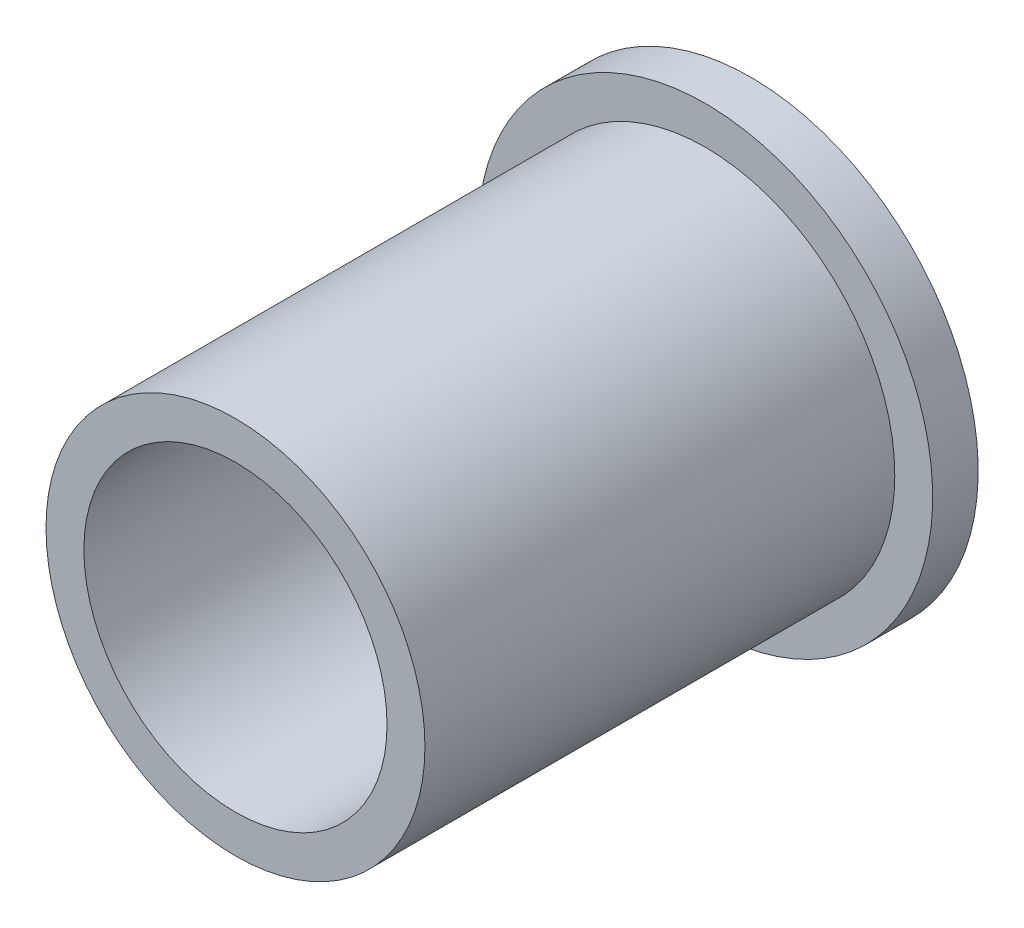
SolidWorks part; units mm, degrees
material "Plain Carbon Steel"
ref_plane "Front Plane" through (0, 0, 0) normal (0, 0, 1) x (1, 0, 0)
ref_plane "Top Plane" through (0, 0, 0) normal (0, 1, 0) x (1, 0, 0)
ref_plane "Right Plane" through (0, 0, 0) normal (1, 0, 0) x (0, 0, -1)
sketch "Body Profile Ø25" plane through (0, 0, 0) normal (0, 0, 1) x (1, 0, 0)
  circle A0 centre (0, 0) radius 12.5
  dimension "D1" = 25
extrude "Bush Body Ø25x31" add sketch "Body Profile Ø25" along normal blind 31
sketch "Flange Profile Ø30" plane through (0, 0, 0) normal (0, 0, -1) x (-1, 0, 0)
  circle A0 centre (0, 0) radius 15
  dimension "D1" = 30
extrude "Flange Ø30x3" add sketch "Flange Profile Ø30" along normal blind 3
sketch "Bore Profile Ø20" plane through (0, 0, -3) normal (0, 0, -1) x (-1, 0, 0)
  circle A0 centre (0, 0) radius 10
  dimension "D1" = 20
extrude "Bore Ø20 Through" cut sketch "Bore Profile Ø20" against normal through all both and the other way through all
